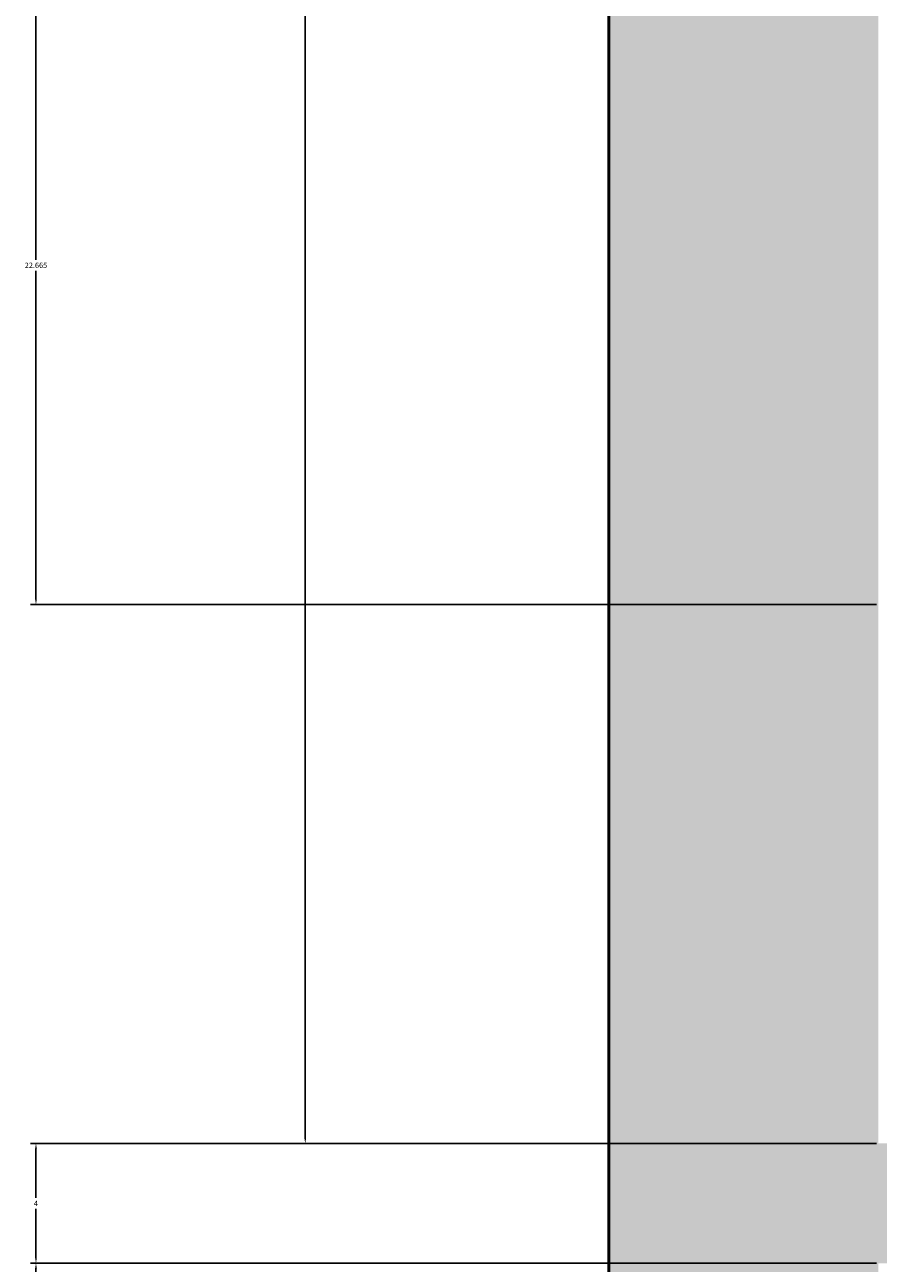
# Model space of a CAD drawing. Units: inches. Extents: x 2307 to 2544, y 2171 to 2540.
# Tile 16 of 52: x 2307 to 2336, y 2388 to 2429. Entities that reach past the tile are written whole.
import ezdxf

# ---------------------------------------------------------------- set-up
doc = ezdxf.new("R2010")
doc.units = ezdxf.units.IN
doc.layers.add('A-ANNO-DIMS', color=2, linetype='Continuous', lineweight=18)
doc.layers.add('A-WALL', color=7, linetype='Continuous', lineweight=50)
doc.layers.add('A-WALL-PATT', color=18, linetype='Continuous', lineweight=13, true_color=0x000000)
doc.styles.get("Standard").update_dxf_attribs({"font": 'arial.ttf'})
doc.dimstyles.get("Standard").update_dxf_attribs({"dimtxt": 0.18, "dimasz": 0.18, "dimexe": 0.18, "dimexo": 0.0625, "dimgap": 0.09, "dimtad": 0, "dimtih": 1, "dimtoh": 1, "dimdec": 4, "dimzin": 0, "dimdsep": 46, "dimtxsty": 'Standard', "dimcen": 0.09, "dimadec": 0, "dimazin": 0, "dimtfac": 1, "dimtdec": 4, "dimtofl": 0, "dimtmove": 0, "dimatfit": 3, "dimfxl": 1, "dimtolj": 1, "dimtzin": 0, "dimarcsym": 0})

# ---------------------------------------------------------------- blocks, each defined once
blk = doc.blocks.new('*D41')
at = {"layer": 'A-ANNO-DIMS', "color": 0, "lineweight": -2, "transparency": 16777216}
for p, q in [((2335.633, 2387.51), (2307.366, 2387.51)), ((2307.546, 2387.33), (2307.546, 2371.636)), ((2307.546, 2355.578), (2307.546, 2371.272)), ((2326.633, 2355.398), (2307.366, 2355.398))]:
    blk.add_line(p, q, dxfattribs=at)
at = {"layer": 'A-ANNO-DIMS', "color": 0, "transparency": 16777216}
for points in [[(2307.516, 2387.33), (2307.576, 2387.33), (2307.546, 2387.51)], [(2307.516, 2355.578), (2307.576, 2355.578), (2307.546, 2355.398)]]:
    blk.add_solid(points, dxfattribs=at)
at = {"layer": 'Defpoints', "color": 0, "transparency": 16777216}
for p in [(2307.546, 2387.51), (2335.696, 2387.51), (2326.696, 2355.398)]:
    blk.add_point(p, dxfattribs=at)
at = {"layer": 'A-ANNO-DIMS', "color": 0, "transparency": 16777216, "insert": (2307.546, 2371.454), "char_height": 0.18, "attachment_point": 5}
blk.add_mtext('\\A1;32.11', dxfattribs=at)
blk = doc.blocks.new('*D47')
at = {"layer": 'A-ANNO-DIMS', "color": 0, "lineweight": -2, "transparency": 16777216}
for p, q in [((2335.633, 2511.51), (2316.366, 2511.51)), ((2316.546, 2511.33), (2316.546, 2451.691)), ((2316.546, 2391.69), (2316.546, 2451.328)), ((2335.633, 2391.51), (2316.366, 2391.51))]:
    blk.add_line(p, q, dxfattribs=at)
at = {"layer": 'A-ANNO-DIMS', "color": 0, "transparency": 16777216}
for points in [[(2316.516, 2511.33), (2316.576, 2511.33), (2316.546, 2511.51)], [(2316.516, 2391.69), (2316.576, 2391.69), (2316.546, 2391.51)]]:
    blk.add_solid(points, dxfattribs=at)
at = {"layer": 'Defpoints', "color": 0, "transparency": 16777216}
for p in [(2316.546, 2511.51), (2335.696, 2511.51), (2335.696, 2391.51)]:
    blk.add_point(p, dxfattribs=at)
at = {"layer": 'A-ANNO-DIMS', "color": 0, "transparency": 16777216, "insert": (2316.546, 2451.51), "char_height": 0.18, "attachment_point": 5}
blk.add_mtext('\\A1;120', dxfattribs=at)
blk = doc.blocks.new('*D50')
at = {"layer": 'A-ANNO-DIMS', "color": 0, "lineweight": -2, "transparency": 16777216}
for p, q in [((2335.633338, 2391.509562), (2307.365838, 2391.509562)), ((2307.545838, 2391.329562), (2307.545838, 2389.689562)), ((2307.545838, 2387.689562), (2307.545838, 2389.329562)), ((2335.633338, 2387.509562), (2307.365838, 2387.509562))]:
    blk.add_line(p, q, dxfattribs=at)
at = {"layer": 'A-ANNO-DIMS', "color": 0, "transparency": 16777216}
for points in [[(2307.515838, 2391.329562), (2307.575838, 2391.329562), (2307.545838, 2391.509562)], [(2307.515838, 2387.689562), (2307.575838, 2387.689562), (2307.545838, 2387.509562)]]:
    blk.add_solid(points, dxfattribs=at)
at = {"layer": 'Defpoints', "color": 0, "transparency": 16777216}
for p in [(2307.545838, 2391.509562), (2335.695838, 2391.509562), (2335.695838, 2387.509562)]:
    blk.add_point(p, dxfattribs=at)
at = {"layer": 'A-ANNO-DIMS', "color": 0, "transparency": 16777216, "insert": (2307.545838, 2389.509562), "char_height": 0.18, "attachment_point": 5}
blk.add_mtext('\\A1;4', dxfattribs=at)
blk = doc.blocks.new('*D67')
at = {"layer": 'A-ANNO-DIMS', "color": 0, "lineweight": -2, "transparency": 16777216}
for p, q in [((2339.646, 2432.174), (2307.366, 2432.174)), ((2307.546, 2431.994), (2307.546, 2421.024)), ((2307.546, 2409.69), (2307.546, 2420.66)), ((2335.633, 2409.51), (2307.366, 2409.51))]:
    blk.add_line(p, q, dxfattribs=at)
at = {"layer": 'A-ANNO-DIMS', "color": 0, "transparency": 16777216}
for points in [[(2307.516, 2431.994), (2307.576, 2431.994), (2307.546, 2432.174)], [(2307.516, 2409.69), (2307.576, 2409.69), (2307.546, 2409.51)]]:
    blk.add_solid(points, dxfattribs=at)
at = {"layer": 'Defpoints', "color": 0, "transparency": 16777216}
for p in [(2307.546, 2432.174), (2339.708, 2432.174), (2335.696, 2409.51)]:
    blk.add_point(p, dxfattribs=at)
at = {"layer": 'A-ANNO-DIMS', "color": 0, "transparency": 16777216, "insert": (2307.546, 2420.842), "char_height": 0.18, "attachment_point": 5}
blk.add_mtext('\\A1;22.665', dxfattribs=at)

msp = doc.modelspace()

# ---------------------------------------------------------------- hatches: boundary and pattern name
at = {"layer": 'A-WALL-PATT'}
h = msp.add_hatch(color=256, dxfattribs=at)
h.dxf.hatch_style = 1
h.paths.add_polyline_path([(2367.4028, 2520.5096), (2326.6958, 2520.5096), (2326.6958, 2355.3983), (2335.6958, 2355.3983), (2335.6958, 2387.5096), (2415.6958, 2387.5096), (2415.6958, 2391.5096), (2335.6958, 2391.5096), (2335.6958, 2409.5096), (2335.6958, 2511.5096), (2367.4028, 2511.5096)])

# ---------------------------------------------------------------- linework, layer by layer
at = {"layer": 'A-WALL'}
msp.add_lwpolyline([(2433.7832, 2190.5096), (2326.6958, 2190.5096), (2326.6958, 2520.5096), (2524.6958, 2520.5096), (2524.6958, 2190.5096), (2469.785, 2190.5096)], dxfattribs=at)

# ---------------------------------------------------------------- dimensions: what is measured, and where the dimension line sits
at = {"layer": 'A-ANNO-DIMS'}
for base, p1, p2, override, picture, middle in [((2316.5458, 2511.5096), (2335.6958, 2391.5096), (2335.6958, 2511.5096), {"dimdec": 0, "dimlfac": 1, "dimrnd": 0, "dimzin": 0, "dimdsep": 46, "dimlunit": 2}, '*D47', (2316.5458, 2451.5096)), ((2307.5458, 2432.1742), (2335.6958, 2409.5096), (2339.7083, 2432.1742), {"dimdec": 3, "dimlfac": 1, "dimrnd": 0, "dimzin": 0, "dimdsep": 46, "dimlunit": 2}, '*D67', (2307.5458, 2420.8419)), ((2307.5458, 2391.5096), (2335.6958, 2387.5096), (2335.6958, 2391.5096), {"dimdec": 0, "dimlfac": 1, "dimrnd": 0, "dimzin": 0, "dimdsep": 46, "dimlunit": 2}, '*D50', (2307.5458, 2389.5096)), ((2307.5458, 2387.5096), (2326.6958, 2355.3983), (2335.6958, 2387.5096), {"dimdec": 2, "dimlfac": 1, "dimrnd": 0, "dimzin": 0, "dimdsep": 46, "dimlunit": 2}, '*D41', (2307.5458, 2371.4539))]:
    dim = msp.add_linear_dim(base=base, p1=p1, p2=p2, angle=90, dimstyle='Standard', override=override, dxfattribs=at)
    dim.commit()
    dim.dimension.update_dxf_attribs({"geometry": picture, "text_midpoint": middle})

doc.saveas('drawing.dxf')
